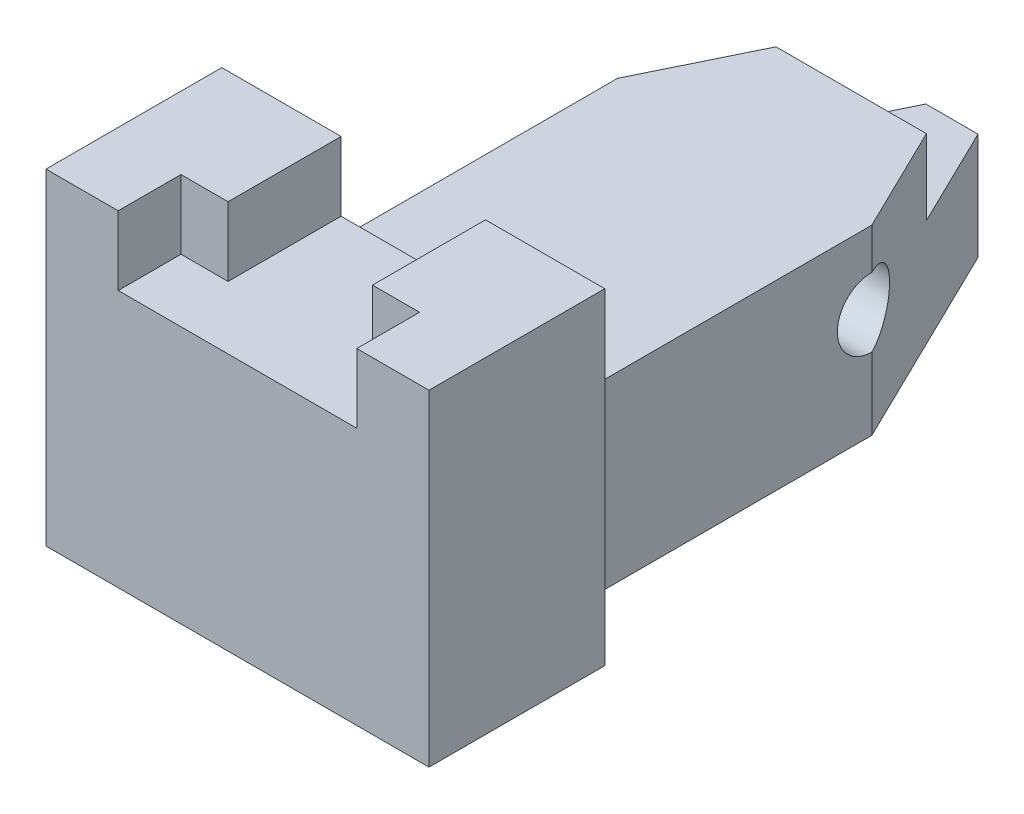
ISO-10303-21;
HEADER;
FILE_DESCRIPTION(('STEP AP214'),'2;1');
FILE_NAME('part.step','',(''),(''),'','','');
FILE_SCHEMA(('AUTOMOTIVE_DESIGN { 1 0 10303 214 1 1 1 1 }'));
ENDSEC;
DATA;
#1=APPLICATION_CONTEXT('core data for automotive mechanical design processes');
#2=APPLICATION_PROTOCOL_DEFINITION('international standard','automotive_design',2000,#1);
#3=PRODUCT_CONTEXT('',#1,'mechanical');
#4=PRODUCT('Part','Part','',(#3));
#5=PRODUCT_RELATED_PRODUCT_CATEGORY('part','',(#4));
#6=PRODUCT_DEFINITION_FORMATION('','',#4);
#7=PRODUCT_DEFINITION_CONTEXT('part definition',#1,'design');
#8=PRODUCT_DEFINITION('design','',#6,#7);
#9=PRODUCT_DEFINITION_SHAPE('','',#8);
#10=(LENGTH_UNIT() NAMED_UNIT(*) SI_UNIT(.MILLI.,.METRE.));
#11=(NAMED_UNIT(*) PLANE_ANGLE_UNIT() SI_UNIT($,.RADIAN.));
#12=(NAMED_UNIT(*) SI_UNIT($,.STERADIAN.) SOLID_ANGLE_UNIT());
#13=UNCERTAINTY_MEASURE_WITH_UNIT(LENGTH_MEASURE(1.E-05),#10,'distance_accuracy_value','');
#14=(GEOMETRIC_REPRESENTATION_CONTEXT(3) GLOBAL_UNCERTAINTY_ASSIGNED_CONTEXT((#13)) GLOBAL_UNIT_ASSIGNED_CONTEXT((#10,
#11,#12)) REPRESENTATION_CONTEXT('',''));
#15=CARTESIAN_POINT('',(0.,0.,0.));
#16=DIRECTION('',(0.,0.,1.));
#17=DIRECTION('',(1.,0.,0.));
#18=AXIS2_PLACEMENT_3D('',#15,#16,#17);
#19=CARTESIAN_POINT('',(-30.5,20.5,120.));
#20=DIRECTION('',(1.,0.,0.));
#21=DIRECTION('',(0.,1.,0.));
#22=AXIS2_PLACEMENT_3D('',#19,#20,#21);
#23=PLANE('',#22);
#24=DIRECTION('',(0.,1.,0.));
#25=VECTOR('',#24,1.);
#26=CARTESIAN_POINT('',(-30.5,20.5,92.));
#27=LINE('',#26,#25);
#28=CARTESIAN_POINT('',(-30.5,-20.5,92.));
#29=VERTEX_POINT('',#28);
#30=CARTESIAN_POINT('',(-30.5,31.5,92.));
#31=VERTEX_POINT('',#30);
#32=EDGE_CURVE('E341',#29,#31,#27,.T.);
#33=ORIENTED_EDGE('',*,*,#32,.F.);
#34=DIRECTION('',(0.,0.,-1.));
#35=VECTOR('',#34,1.);
#36=CARTESIAN_POINT('',(-30.5,-20.5,120.));
#37=LINE('',#36,#35);
#38=CARTESIAN_POINT('',(-30.5,-20.5,120.));
#39=VERTEX_POINT('',#38);
#40=EDGE_CURVE('E339',#39,#29,#37,.T.);
#41=ORIENTED_EDGE('',*,*,#40,.F.);
#42=DIRECTION('',(0.,-1.,0.));
#43=VECTOR('',#42,1.);
#44=CARTESIAN_POINT('',(-30.5,20.5,120.));
#45=LINE('',#44,#43);
#46=CARTESIAN_POINT('',(-30.5,31.5,120.));
#47=VERTEX_POINT('',#46);
#48=EDGE_CURVE('E335',#47,#39,#45,.T.);
#49=ORIENTED_EDGE('',*,*,#48,.F.);
#50=DIRECTION('',(0.,0.,1.));
#51=VECTOR('',#50,1.);
#52=CARTESIAN_POINT('',(-30.5,31.5,120.));
#53=LINE('',#52,#51);
#54=EDGE_CURVE('E254',#31,#47,#53,.T.);
#55=ORIENTED_EDGE('',*,*,#54,.F.);
#56=EDGE_LOOP('',(#33,#41,#49,#55));
#57=FACE_BOUND('',#56,.T.);
#58=ADVANCED_FACE('F41',(#57),#23,.F.);
#59=CARTESIAN_POINT('',(30.5,20.5,120.));
#60=DIRECTION('',(-1.,0.,0.));
#61=DIRECTION('',(0.,-1.,0.));
#62=AXIS2_PLACEMENT_3D('',#59,#60,#61);
#63=PLANE('',#62);
#64=DIRECTION('',(0.,0.,-1.));
#65=VECTOR('',#64,1.);
#66=CARTESIAN_POINT('',(30.5,-20.5,120.));
#67=LINE('',#66,#65);
#68=CARTESIAN_POINT('',(30.5,-20.5,120.));
#69=VERTEX_POINT('',#68);
#70=CARTESIAN_POINT('',(30.5,-20.5,92.));
#71=VERTEX_POINT('',#70);
#72=EDGE_CURVE('E337',#69,#71,#67,.T.);
#73=ORIENTED_EDGE('',*,*,#72,.T.);
#74=DIRECTION('',(0.,1.,0.));
#75=VECTOR('',#74,1.);
#76=CARTESIAN_POINT('',(30.5,0.,92.));
#77=LINE('',#76,#75);
#78=CARTESIAN_POINT('',(30.5,31.5,92.));
#79=VERTEX_POINT('',#78);
#80=EDGE_CURVE('E278',#71,#79,#77,.T.);
#81=ORIENTED_EDGE('',*,*,#80,.T.);
#82=DIRECTION('',(0.,0.,-1.));
#83=VECTOR('',#82,1.);
#84=CARTESIAN_POINT('',(30.5,31.5,92.));
#85=LINE('',#84,#83);
#86=CARTESIAN_POINT('',(30.5,31.5,120.));
#87=VERTEX_POINT('',#86);
#88=EDGE_CURVE('E305',#87,#79,#85,.T.);
#89=ORIENTED_EDGE('',*,*,#88,.F.);
#90=DIRECTION('',(0.,1.,0.));
#91=VECTOR('',#90,1.);
#92=CARTESIAN_POINT('',(30.5,20.5,120.));
#93=LINE('',#92,#91);
#94=EDGE_CURVE('E316',#69,#87,#93,.T.);
#95=ORIENTED_EDGE('',*,*,#94,.F.);
#96=EDGE_LOOP('',(#73,#81,#89,#95));
#97=FACE_BOUND('',#96,.T.);
#98=ADVANCED_FACE('F43',(#97),#63,.F.);
#99=CARTESIAN_POINT('',(-89.5,0.,22.));
#100=DIRECTION('',(0.,0.,-1.));
#101=DIRECTION('',(-1.,0.,0.));
#102=AXIS2_PLACEMENT_3D('',#99,#100,#101);
#103=PLANE('',#102);
#104=DIRECTION('',(1.,0.,0.));
#105=VECTOR('',#104,1.);
#106=CARTESIAN_POINT('',(-89.5,-3.50000000000002,22.));
#107=LINE('',#106,#105);
#108=CARTESIAN_POINT('',(-12.2301169484492,-3.50000000000001,22.));
#109=VERTEX_POINT('',#108);
#110=CARTESIAN_POINT('',(11.7239944957032,-3.50000000000001,22.));
#111=VERTEX_POINT('',#110);
#112=EDGE_CURVE('E318',#109,#111,#107,.T.);
#113=ORIENTED_EDGE('',*,*,#112,.F.);
#114=DIRECTION('',(0.,1.,0.));
#115=VECTOR('',#114,1.);
#116=CARTESIAN_POINT('',(-12.2301169484492,0.,22.));
#117=LINE('',#116,#115);
#118=CARTESIAN_POINT('',(-12.2301169484492,8.49999999999999,22.));
#119=VERTEX_POINT('',#118);
#120=EDGE_CURVE('E234',#109,#119,#117,.T.);
#121=ORIENTED_EDGE('',*,*,#120,.T.);
#122=DIRECTION('',(1.,0.,0.));
#123=VECTOR('',#122,1.);
#124=CARTESIAN_POINT('',(-89.5,8.49999999999998,22.));
#125=LINE('',#124,#123);
#126=CARTESIAN_POINT('',(11.7239944957032,8.5,22.));
#127=VERTEX_POINT('',#126);
#128=EDGE_CURVE('E325',#119,#127,#125,.T.);
#129=ORIENTED_EDGE('',*,*,#128,.T.);
#130=DIRECTION('',(0.,-1.,0.));
#131=VECTOR('',#130,1.);
#132=CARTESIAN_POINT('',(11.7239944957032,0.,22.));
#133=LINE('',#132,#131);
#134=EDGE_CURVE('E225',#127,#111,#133,.T.);
#135=ORIENTED_EDGE('',*,*,#134,.T.);
#136=EDGE_LOOP('',(#113,#121,#129,#135));
#137=FACE_BOUND('',#136,.T.);
#138=ADVANCED_FACE('F413',(#137),#103,.T.);
#139=CARTESIAN_POINT('',(-89.5,8.49999999999998,0.));
#140=DIRECTION('',(0.,1.,0.));
#141=DIRECTION('',(-1.,0.,0.));
#142=AXIS2_PLACEMENT_3D('',#139,#140,#141);
#143=PLANE('',#142);
#144=ORIENTED_EDGE('',*,*,#128,.F.);
#145=DIRECTION('',(-0.438371146789085,0.,0.898794046299164));
#146=VECTOR('',#145,1.);
#147=CARTESIAN_POINT('',(-18.4108950856716,8.49999999999999,34.6724731586962));
#148=LINE('',#147,#146);
#149=CARTESIAN_POINT('',(-20.5,8.49999999999999,38.9557729900058));
#150=VERTEX_POINT('',#149);
#151=EDGE_CURVE('E353',#119,#150,#148,.T.);
#152=ORIENTED_EDGE('',*,*,#151,.T.);
#153=DIRECTION('',(0.,0.,-1.));
#154=VECTOR('',#153,1.);
#155=CARTESIAN_POINT('',(-20.5,8.49999999999999,0.));
#156=LINE('',#155,#154);
#157=CARTESIAN_POINT('',(-20.5,8.49999999999998,92.));
#158=VERTEX_POINT('',#157);
#159=EDGE_CURVE('E198',#158,#150,#156,.T.);
#160=ORIENTED_EDGE('',*,*,#159,.F.);
#161=DIRECTION('',(1.,0.,0.));
#162=VECTOR('',#161,1.);
#163=CARTESIAN_POINT('',(-89.5,8.49999999999997,92.));
#164=LINE('',#163,#162);
#165=CARTESIAN_POINT('',(19.9938775472544,8.49999999999999,92.));
#166=VERTEX_POINT('',#165);
#167=EDGE_CURVE('E314',#158,#166,#164,.T.);
#168=ORIENTED_EDGE('',*,*,#167,.T.);
#169=DIRECTION('',(0.,0.,1.));
#170=VECTOR('',#169,1.);
#171=CARTESIAN_POINT('',(19.9938775472544,8.5,0.));
#172=LINE('',#171,#170);
#173=CARTESIAN_POINT('',(19.9938775472544,8.49999999999999,38.9557729900071));
#174=VERTEX_POINT('',#173);
#175=EDGE_CURVE('E342',#174,#166,#172,.T.);
#176=ORIENTED_EDGE('',*,*,#175,.F.);
#177=DIRECTION('',(-0.438371146789072,0.,-0.89879404629917));
#178=VECTOR('',#177,1.);
#179=CARTESIAN_POINT('',(-16.3962641470313,8.5,-35.6550743214029));
#180=LINE('',#179,#178);
#181=EDGE_CURVE('E350',#174,#127,#180,.T.);
#182=ORIENTED_EDGE('',*,*,#181,.T.);
#183=EDGE_LOOP('',(#144,#152,#160,#168,#176,#182));
#184=FACE_BOUND('',#183,.T.);
#185=ADVANCED_FACE('F407',(#184),#143,.T.);
#186=CARTESIAN_POINT('',(-30.5,20.5,120.));
#187=DIRECTION('',(0.,-1.,0.));
#188=DIRECTION('',(0.,0.,-1.));
#189=AXIS2_PLACEMENT_3D('',#186,#187,#188);
#190=PLANE('',#189);
#191=DIRECTION('',(0.,0.,-1.));
#192=VECTOR('',#191,1.);
#193=CARTESIAN_POINT('',(-19.,20.5,110.));
#194=LINE('',#193,#192);
#195=CARTESIAN_POINT('',(-19.,20.5,120.));
#196=VERTEX_POINT('',#195);
#197=CARTESIAN_POINT('',(-19.,20.5,110.));
#198=VERTEX_POINT('',#197);
#199=EDGE_CURVE('E258',#196,#198,#194,.T.);
#200=ORIENTED_EDGE('',*,*,#199,.F.);
#201=DIRECTION('',(-1.,0.,0.));
#202=VECTOR('',#201,1.);
#203=CARTESIAN_POINT('',(-30.5,20.5,120.));
#204=LINE('',#203,#202);
#205=CARTESIAN_POINT('',(19.,20.5,120.));
#206=VERTEX_POINT('',#205);
#207=EDGE_CURVE('E326',#206,#196,#204,.T.);
#208=ORIENTED_EDGE('',*,*,#207,.F.);
#209=DIRECTION('',(0.,0.,1.));
#210=VECTOR('',#209,1.);
#211=CARTESIAN_POINT('',(19.,20.5,120.));
#212=LINE('',#211,#210);
#213=CARTESIAN_POINT('',(19.,20.5,110.));
#214=VERTEX_POINT('',#213);
#215=EDGE_CURVE('E292',#214,#206,#212,.T.);
#216=ORIENTED_EDGE('',*,*,#215,.F.);
#217=DIRECTION('',(1.,0.,0.));
#218=VECTOR('',#217,1.);
#219=CARTESIAN_POINT('',(19.,20.5,110.));
#220=LINE('',#219,#218);
#221=CARTESIAN_POINT('',(11.5,20.5,110.));
#222=VERTEX_POINT('',#221);
#223=EDGE_CURVE('E294',#222,#214,#220,.T.);
#224=ORIENTED_EDGE('',*,*,#223,.F.);
#225=DIRECTION('',(0.,0.,1.));
#226=VECTOR('',#225,1.);
#227=CARTESIAN_POINT('',(11.5,20.5,110.));
#228=LINE('',#227,#226);
#229=CARTESIAN_POINT('',(11.5,20.5,92.));
#230=VERTEX_POINT('',#229);
#231=EDGE_CURVE('E264',#230,#222,#228,.T.);
#232=ORIENTED_EDGE('',*,*,#231,.F.);
#233=DIRECTION('',(1.,0.,0.));
#234=VECTOR('',#233,1.);
#235=CARTESIAN_POINT('',(-89.5,20.5,92.));
#236=LINE('',#235,#234);
#237=CARTESIAN_POINT('',(-11.5,20.5,92.));
#238=VERTEX_POINT('',#237);
#239=EDGE_CURVE('E317',#238,#230,#236,.T.);
#240=ORIENTED_EDGE('',*,*,#239,.F.);
#241=DIRECTION('',(0.,0.,-1.));
#242=VECTOR('',#241,1.);
#243=CARTESIAN_POINT('',(-11.5,20.5,92.));
#244=LINE('',#243,#242);
#245=CARTESIAN_POINT('',(-11.5,20.5,110.));
#246=VERTEX_POINT('',#245);
#247=EDGE_CURVE('E250',#246,#238,#244,.T.);
#248=ORIENTED_EDGE('',*,*,#247,.F.);
#249=DIRECTION('',(1.,0.,0.));
#250=VECTOR('',#249,1.);
#251=CARTESIAN_POINT('',(-11.5,20.5,110.));
#252=LINE('',#251,#250);
#253=EDGE_CURVE('E265',#198,#246,#252,.T.);
#254=ORIENTED_EDGE('',*,*,#253,.F.);
#255=EDGE_LOOP('',(#200,#208,#216,#224,#232,#240,#248,#254));
#256=FACE_BOUND('',#255,.T.);
#257=ADVANCED_FACE('F437',(#256),#190,.F.);
#258=CARTESIAN_POINT('',(-30.5,-20.5,120.));
#259=DIRECTION('',(0.,1.,0.));
#260=DIRECTION('',(0.,0.,1.));
#261=AXIS2_PLACEMENT_3D('',#258,#259,#260);
#262=PLANE('',#261);
#263=DIRECTION('',(-0.438371146789085,0.,0.898794046299164));
#264=VECTOR('',#263,1.);
#265=CARTESIAN_POINT('',(-54.353553824182,-20.5,108.365844446836));
#266=LINE('',#265,#264);
#267=CARTESIAN_POINT('',(-4.40482457732624,-20.5,5.95577299000578));
#268=VERTEX_POINT('',#267);
#269=CARTESIAN_POINT('',(-20.5,-20.5,38.9557729900058));
#270=VERTEX_POINT('',#269);
#271=EDGE_CURVE('E239',#268,#270,#266,.T.);
#272=ORIENTED_EDGE('',*,*,#271,.F.);
#273=DIRECTION('',(1.,0.,0.));
#274=VECTOR('',#273,1.);
#275=CARTESIAN_POINT('',(-30.4999999999997,-20.5,5.95577299000573));
#276=LINE('',#275,#274);
#277=CARTESIAN_POINT('',(3.89870212458057,-20.5,5.9557729900058));
#278=VERTEX_POINT('',#277);
#279=EDGE_CURVE('E47',#268,#278,#276,.T.);
#280=ORIENTED_EDGE('',*,*,#279,.T.);
#281=DIRECTION('',(-0.438371146789072,0.,-0.89879404629917));
#282=VECTOR('',#281,1.);
#283=CARTESIAN_POINT('',(42.2223675472644,-20.5,84.5309314295353));
#284=LINE('',#283,#282);
#285=CARTESIAN_POINT('',(19.9938775472544,-20.5,38.9557729900071));
#286=VERTEX_POINT('',#285);
#287=EDGE_CURVE('E226',#286,#278,#284,.T.);
#288=ORIENTED_EDGE('',*,*,#287,.F.);
#289=DIRECTION('',(0.,0.,1.));
#290=VECTOR('',#289,1.);
#291=CARTESIAN_POINT('',(19.9938775472544,-20.5,120.));
#292=LINE('',#291,#290);
#293=CARTESIAN_POINT('',(19.9938775472544,-20.5,92.));
#294=VERTEX_POINT('',#293);
#295=EDGE_CURVE('E216',#286,#294,#292,.T.);
#296=ORIENTED_EDGE('',*,*,#295,.T.);
#297=DIRECTION('',(-1.,0.,0.));
#298=VECTOR('',#297,1.);
#299=CARTESIAN_POINT('',(-30.5,-20.5,92.));
#300=LINE('',#299,#298);
#301=EDGE_CURVE('E351',#71,#294,#300,.T.);
#302=ORIENTED_EDGE('',*,*,#301,.F.);
#303=ORIENTED_EDGE('',*,*,#72,.F.);
#304=DIRECTION('',(1.,0.,0.));
#305=VECTOR('',#304,1.);
#306=CARTESIAN_POINT('',(-30.5,-20.5,120.));
#307=LINE('',#306,#305);
#308=EDGE_CURVE('E334',#39,#69,#307,.T.);
#309=ORIENTED_EDGE('',*,*,#308,.F.);
#310=ORIENTED_EDGE('',*,*,#40,.T.);
#311=DIRECTION('',(-1.,0.,0.));
#312=VECTOR('',#311,1.);
#313=CARTESIAN_POINT('',(-30.5,-20.5,92.));
#314=LINE('',#313,#312);
#315=CARTESIAN_POINT('',(-20.5,-20.5,92.));
#316=VERTEX_POINT('',#315);
#317=EDGE_CURVE('E352',#316,#29,#314,.T.);
#318=ORIENTED_EDGE('',*,*,#317,.F.);
#319=DIRECTION('',(0.,0.,-1.));
#320=VECTOR('',#319,1.);
#321=CARTESIAN_POINT('',(-20.5,-20.5,120.));
#322=LINE('',#321,#320);
#323=EDGE_CURVE('E233',#316,#270,#322,.T.);
#324=ORIENTED_EDGE('',*,*,#323,.T.);
#325=EDGE_LOOP('',(#272,#280,#288,#296,#302,#303,#309,#310,#318,#324));
#326=FACE_BOUND('',#325,.T.);
#327=ADVANCED_FACE('F363',(#326),#262,.F.);
#328=CARTESIAN_POINT('',(0.,0.,120.));
#329=DIRECTION('',(0.,0.,1.));
#330=DIRECTION('',(1.,0.,0.));
#331=AXIS2_PLACEMENT_3D('',#328,#329,#330);
#332=PLANE('',#331);
#333=ORIENTED_EDGE('',*,*,#94,.T.);
#334=DIRECTION('',(1.,0.,0.));
#335=VECTOR('',#334,1.);
#336=CARTESIAN_POINT('',(30.5,31.5,120.));
#337=LINE('',#336,#335);
#338=CARTESIAN_POINT('',(19.,31.5,120.));
#339=VERTEX_POINT('',#338);
#340=EDGE_CURVE('E304',#339,#87,#337,.T.);
#341=ORIENTED_EDGE('',*,*,#340,.F.);
#342=DIRECTION('',(0.,-1.,0.));
#343=VECTOR('',#342,1.);
#344=CARTESIAN_POINT('',(19.,31.5,120.));
#345=LINE('',#344,#343);
#346=EDGE_CURVE('E283',#339,#206,#345,.T.);
#347=ORIENTED_EDGE('',*,*,#346,.T.);
#348=ORIENTED_EDGE('',*,*,#207,.T.);
#349=DIRECTION('',(0.,-1.,0.));
#350=VECTOR('',#349,1.);
#351=CARTESIAN_POINT('',(-19.,31.5,120.));
#352=LINE('',#351,#350);
#353=CARTESIAN_POINT('',(-19.,31.5,120.));
#354=VERTEX_POINT('',#353);
#355=EDGE_CURVE('E260',#354,#196,#352,.T.);
#356=ORIENTED_EDGE('',*,*,#355,.F.);
#357=DIRECTION('',(1.,0.,0.));
#358=VECTOR('',#357,1.);
#359=CARTESIAN_POINT('',(-19.,31.5,120.));
#360=LINE('',#359,#358);
#361=EDGE_CURVE('E259',#47,#354,#360,.T.);
#362=ORIENTED_EDGE('',*,*,#361,.F.);
#363=ORIENTED_EDGE('',*,*,#48,.T.);
#364=ORIENTED_EDGE('',*,*,#308,.T.);
#365=EDGE_LOOP('',(#333,#341,#347,#348,#356,#362,#363,#364));
#366=FACE_BOUND('',#365,.T.);
#367=ADVANCED_FACE('F382',(#366),#332,.T.);
#368=CARTESIAN_POINT('',(-89.5,0.,92.));
#369=DIRECTION('',(0.,0.,-1.));
#370=DIRECTION('',(-1.,0.,0.));
#371=AXIS2_PLACEMENT_3D('',#368,#369,#370);
#372=PLANE('',#371);
#373=ORIENTED_EDGE('',*,*,#80,.F.);
#374=ORIENTED_EDGE('',*,*,#301,.T.);
#375=DIRECTION('',(0.,-1.,0.));
#376=VECTOR('',#375,1.);
#377=CARTESIAN_POINT('',(19.9938775472544,31.5,92.));
#378=LINE('',#377,#376);
#379=EDGE_CURVE('E208',#166,#294,#378,.T.);
#380=ORIENTED_EDGE('',*,*,#379,.F.);
#381=ORIENTED_EDGE('',*,*,#167,.F.);
#382=DIRECTION('',(0.,1.,0.));
#383=VECTOR('',#382,1.);
#384=CARTESIAN_POINT('',(-20.5,-51.,92.));
#385=LINE('',#384,#383);
#386=EDGE_CURVE('E205',#316,#158,#385,.T.);
#387=ORIENTED_EDGE('',*,*,#386,.F.);
#388=ORIENTED_EDGE('',*,*,#317,.T.);
#389=ORIENTED_EDGE('',*,*,#32,.T.);
#390=DIRECTION('',(-1.,0.,0.));
#391=VECTOR('',#390,1.);
#392=CARTESIAN_POINT('',(-30.5,31.5,92.));
#393=LINE('',#392,#391);
#394=CARTESIAN_POINT('',(-11.5,31.5,92.));
#395=VERTEX_POINT('',#394);
#396=EDGE_CURVE('E252',#395,#31,#393,.T.);
#397=ORIENTED_EDGE('',*,*,#396,.F.);
#398=DIRECTION('',(0.,-1.,0.));
#399=VECTOR('',#398,1.);
#400=CARTESIAN_POINT('',(-11.5,31.5,92.));
#401=LINE('',#400,#399);
#402=EDGE_CURVE('E267',#395,#238,#401,.T.);
#403=ORIENTED_EDGE('',*,*,#402,.T.);
#404=ORIENTED_EDGE('',*,*,#239,.T.);
#405=DIRECTION('',(0.,-1.,0.));
#406=VECTOR('',#405,1.);
#407=CARTESIAN_POINT('',(11.5,31.5,92.));
#408=LINE('',#407,#406);
#409=CARTESIAN_POINT('',(11.5,31.5,92.));
#410=VERTEX_POINT('',#409);
#411=EDGE_CURVE('E286',#410,#230,#408,.T.);
#412=ORIENTED_EDGE('',*,*,#411,.F.);
#413=DIRECTION('',(-1.,0.,0.));
#414=VECTOR('',#413,1.);
#415=CARTESIAN_POINT('',(11.5,31.5,92.));
#416=LINE('',#415,#414);
#417=EDGE_CURVE('E293',#79,#410,#416,.T.);
#418=ORIENTED_EDGE('',*,*,#417,.F.);
#419=EDGE_LOOP('',(#373,#374,#380,#381,#387,#388,#389,#397,#403,#404,#412,#418));
#420=FACE_BOUND('',#419,.T.);
#421=ADVANCED_FACE('F403',(#420),#372,.T.);
#422=CARTESIAN_POINT('',(-89.5,-3.50000000000002,0.));
#423=DIRECTION('',(0.,1.,0.));
#424=DIRECTION('',(-1.,0.,0.));
#425=AXIS2_PLACEMENT_3D('',#422,#423,#424);
#426=PLANE('',#425);
#427=DIRECTION('',(1.,0.,0.));
#428=VECTOR('',#427,1.);
#429=CARTESIAN_POINT('',(3.89870212458057,-3.5,5.9557729900058));
#430=LINE('',#429,#428);
#431=CARTESIAN_POINT('',(-4.40482457732625,-3.5,5.95577299000578));
#432=VERTEX_POINT('',#431);
#433=CARTESIAN_POINT('',(3.89870212458057,-3.5,5.9557729900058));
#434=VERTEX_POINT('',#433);
#435=EDGE_CURVE('E202',#432,#434,#430,.T.);
#436=ORIENTED_EDGE('',*,*,#435,.F.);
#437=DIRECTION('',(-0.438371146789085,0.,0.898794046299164));
#438=VECTOR('',#437,1.);
#439=CARTESIAN_POINT('',(-18.4108950856716,-3.50000000000001,34.6724731586962));
#440=LINE('',#439,#438);
#441=EDGE_CURVE('E240',#432,#109,#440,.T.);
#442=ORIENTED_EDGE('',*,*,#441,.T.);
#443=ORIENTED_EDGE('',*,*,#112,.T.);
#444=DIRECTION('',(-0.438371146789072,0.,-0.89879404629917));
#445=VECTOR('',#444,1.);
#446=CARTESIAN_POINT('',(-16.3962641470313,-3.5,-35.6550743214029));
#447=LINE('',#446,#445);
#448=EDGE_CURVE('E222',#111,#434,#447,.T.);
#449=ORIENTED_EDGE('',*,*,#448,.T.);
#450=EDGE_LOOP('',(#436,#442,#443,#449));
#451=FACE_BOUND('',#450,.T.);
#452=ADVANCED_FACE('F416',(#451),#426,.T.);
#453=CARTESIAN_POINT('',(11.5,31.5,110.));
#454=DIRECTION('',(1.,0.,0.));
#455=DIRECTION('',(0.,0.,-1.));
#456=AXIS2_PLACEMENT_3D('',#453,#454,#455);
#457=PLANE('',#456);
#458=ORIENTED_EDGE('',*,*,#231,.T.);
#459=DIRECTION('',(0.,-1.,0.));
#460=VECTOR('',#459,1.);
#461=CARTESIAN_POINT('',(11.5,31.5,110.));
#462=LINE('',#461,#460);
#463=CARTESIAN_POINT('',(11.5,31.5,110.));
#464=VERTEX_POINT('',#463);
#465=EDGE_CURVE('E245',#464,#222,#462,.T.);
#466=ORIENTED_EDGE('',*,*,#465,.F.);
#467=DIRECTION('',(0.,0.,1.));
#468=VECTOR('',#467,1.);
#469=CARTESIAN_POINT('',(11.5,31.5,110.));
#470=LINE('',#469,#468);
#471=EDGE_CURVE('E298',#410,#464,#470,.T.);
#472=ORIENTED_EDGE('',*,*,#471,.F.);
#473=ORIENTED_EDGE('',*,*,#411,.T.);
#474=EDGE_LOOP('',(#458,#466,#472,#473));
#475=FACE_BOUND('',#474,.T.);
#476=ADVANCED_FACE('F457',(#475),#457,.F.);
#477=CARTESIAN_POINT('',(19.,31.5,110.));
#478=DIRECTION('',(0.,0.,-1.));
#479=DIRECTION('',(-1.,0.,0.));
#480=AXIS2_PLACEMENT_3D('',#477,#478,#479);
#481=PLANE('',#480);
#482=ORIENTED_EDGE('',*,*,#223,.T.);
#483=DIRECTION('',(0.,-1.,0.));
#484=VECTOR('',#483,1.);
#485=CARTESIAN_POINT('',(19.,31.5,110.));
#486=LINE('',#485,#484);
#487=CARTESIAN_POINT('',(19.,31.5,110.));
#488=VERTEX_POINT('',#487);
#489=EDGE_CURVE('E285',#488,#214,#486,.T.);
#490=ORIENTED_EDGE('',*,*,#489,.F.);
#491=DIRECTION('',(1.,0.,0.));
#492=VECTOR('',#491,1.);
#493=CARTESIAN_POINT('',(19.,31.5,110.));
#494=LINE('',#493,#492);
#495=EDGE_CURVE('E309',#464,#488,#494,.T.);
#496=ORIENTED_EDGE('',*,*,#495,.F.);
#497=ORIENTED_EDGE('',*,*,#465,.T.);
#498=EDGE_LOOP('',(#482,#490,#496,#497));
#499=FACE_BOUND('',#498,.T.);
#500=ADVANCED_FACE('F456',(#499),#481,.F.);
#501=CARTESIAN_POINT('',(19.,31.5,120.));
#502=DIRECTION('',(1.,0.,0.));
#503=DIRECTION('',(0.,0.,-1.));
#504=AXIS2_PLACEMENT_3D('',#501,#502,#503);
#505=PLANE('',#504);
#506=ORIENTED_EDGE('',*,*,#215,.T.);
#507=ORIENTED_EDGE('',*,*,#346,.F.);
#508=DIRECTION('',(0.,0.,1.));
#509=VECTOR('',#508,1.);
#510=CARTESIAN_POINT('',(19.,31.5,120.));
#511=LINE('',#510,#509);
#512=EDGE_CURVE('E308',#488,#339,#511,.T.);
#513=ORIENTED_EDGE('',*,*,#512,.F.);
#514=ORIENTED_EDGE('',*,*,#489,.T.);
#515=EDGE_LOOP('',(#506,#507,#513,#514));
#516=FACE_BOUND('',#515,.T.);
#517=ADVANCED_FACE('F388',(#516),#505,.F.);
#518=CARTESIAN_POINT('',(0.,31.5,0.));
#519=DIRECTION('',(0.,-1.,0.));
#520=DIRECTION('',(0.,0.,-1.));
#521=AXIS2_PLACEMENT_3D('',#518,#519,#520);
#522=PLANE('',#521);
#523=ORIENTED_EDGE('',*,*,#471,.T.);
#524=ORIENTED_EDGE('',*,*,#495,.T.);
#525=ORIENTED_EDGE('',*,*,#512,.T.);
#526=ORIENTED_EDGE('',*,*,#340,.T.);
#527=ORIENTED_EDGE('',*,*,#88,.T.);
#528=ORIENTED_EDGE('',*,*,#417,.T.);
#529=EDGE_LOOP('',(#523,#524,#525,#526,#527,#528));
#530=FACE_BOUND('',#529,.T.);
#531=ADVANCED_FACE('F384',(#530),#522,.F.);
#532=CARTESIAN_POINT('',(-19.,31.5,110.));
#533=DIRECTION('',(-1.,0.,0.));
#534=DIRECTION('',(0.,0.,1.));
#535=AXIS2_PLACEMENT_3D('',#532,#533,#534);
#536=PLANE('',#535);
#537=ORIENTED_EDGE('',*,*,#199,.T.);
#538=DIRECTION('',(0.,-1.,0.));
#539=VECTOR('',#538,1.);
#540=CARTESIAN_POINT('',(-19.,31.5,110.));
#541=LINE('',#540,#539);
#542=CARTESIAN_POINT('',(-19.,31.5,110.));
#543=VERTEX_POINT('',#542);
#544=EDGE_CURVE('E279',#543,#198,#541,.T.);
#545=ORIENTED_EDGE('',*,*,#544,.F.);
#546=DIRECTION('',(0.,0.,-1.));
#547=VECTOR('',#546,1.);
#548=CARTESIAN_POINT('',(-19.,31.5,110.));
#549=LINE('',#548,#547);
#550=EDGE_CURVE('E243',#354,#543,#549,.T.);
#551=ORIENTED_EDGE('',*,*,#550,.F.);
#552=ORIENTED_EDGE('',*,*,#355,.T.);
#553=EDGE_LOOP('',(#537,#545,#551,#552));
#554=FACE_BOUND('',#553,.T.);
#555=ADVANCED_FACE('F393',(#554),#536,.F.);
#556=CARTESIAN_POINT('',(-11.5,31.5,110.));
#557=DIRECTION('',(0.,0.,-1.));
#558=DIRECTION('',(-1.,0.,0.));
#559=AXIS2_PLACEMENT_3D('',#556,#557,#558);
#560=PLANE('',#559);
#561=ORIENTED_EDGE('',*,*,#253,.T.);
#562=DIRECTION('',(0.,-1.,0.));
#563=VECTOR('',#562,1.);
#564=CARTESIAN_POINT('',(-11.5,31.5,110.));
#565=LINE('',#564,#563);
#566=CARTESIAN_POINT('',(-11.5,31.5,110.));
#567=VERTEX_POINT('',#566);
#568=EDGE_CURVE('E271',#567,#246,#565,.T.);
#569=ORIENTED_EDGE('',*,*,#568,.F.);
#570=DIRECTION('',(1.,0.,0.));
#571=VECTOR('',#570,1.);
#572=CARTESIAN_POINT('',(-11.5,31.5,110.));
#573=LINE('',#572,#571);
#574=EDGE_CURVE('E246',#543,#567,#573,.T.);
#575=ORIENTED_EDGE('',*,*,#574,.F.);
#576=ORIENTED_EDGE('',*,*,#544,.T.);
#577=EDGE_LOOP('',(#561,#569,#575,#576));
#578=FACE_BOUND('',#577,.T.);
#579=ADVANCED_FACE('F449',(#578),#560,.F.);
#580=CARTESIAN_POINT('',(-11.5,31.5,92.));
#581=DIRECTION('',(-1.,0.,0.));
#582=DIRECTION('',(0.,0.,1.));
#583=AXIS2_PLACEMENT_3D('',#580,#581,#582);
#584=PLANE('',#583);
#585=ORIENTED_EDGE('',*,*,#247,.T.);
#586=ORIENTED_EDGE('',*,*,#402,.F.);
#587=DIRECTION('',(0.,0.,-1.));
#588=VECTOR('',#587,1.);
#589=CARTESIAN_POINT('',(-11.5,31.5,92.));
#590=LINE('',#589,#588);
#591=EDGE_CURVE('E248',#567,#395,#590,.T.);
#592=ORIENTED_EDGE('',*,*,#591,.F.);
#593=ORIENTED_EDGE('',*,*,#568,.T.);
#594=EDGE_LOOP('',(#585,#586,#592,#593));
#595=FACE_BOUND('',#594,.T.);
#596=ADVANCED_FACE('F451',(#595),#584,.F.);
#597=CARTESIAN_POINT('',(0.,31.5,0.));
#598=DIRECTION('',(0.,-1.,0.));
#599=DIRECTION('',(0.,0.,-1.));
#600=AXIS2_PLACEMENT_3D('',#597,#598,#599);
#601=PLANE('',#600);
#602=ORIENTED_EDGE('',*,*,#550,.T.);
#603=ORIENTED_EDGE('',*,*,#574,.T.);
#604=ORIENTED_EDGE('',*,*,#591,.T.);
#605=ORIENTED_EDGE('',*,*,#396,.T.);
#606=ORIENTED_EDGE('',*,*,#54,.T.);
#607=ORIENTED_EDGE('',*,*,#361,.T.);
#608=EDGE_LOOP('',(#602,#603,#604,#605,#606,#607));
#609=FACE_BOUND('',#608,.T.);
#610=ADVANCED_FACE('F396',(#609),#601,.F.);
#611=CARTESIAN_POINT('',(0.80288483214509,31.5,-0.391593097502386));
#612=DIRECTION('',(0.89879404629917,0.,-0.438371146789072));
#613=DIRECTION('',(-0.438371146789072,0.,-0.89879404629917));
#614=AXIS2_PLACEMENT_3D('',#611,#612,#613);
#615=PLANE('',#614);
#616=CARTESIAN_POINT('',(19.9938775472544,-3.5,38.9557729900071));
#617=DIRECTION('',(0.89879404629917,0.,-0.438371146789072));
#618=DIRECTION('',(0.438371146789072,0.,0.89879404629917));
#619=AXIS2_PLACEMENT_3D('',#616,#617,#618);
#620=ELLIPSE('',#619,6.11931067261352,5.5);
#621=CARTESIAN_POINT('',(19.9938775472544,-9.,38.9557729900071));
#622=VERTEX_POINT('',#621);
#623=CARTESIAN_POINT('',(19.9938775472544,1.99999999999999,38.9557729900071));
#624=VERTEX_POINT('',#623);
#625=EDGE_CURVE('E54',#622,#624,#620,.T.);
#626=ORIENTED_EDGE('',*,*,#625,.F.);
#627=DIRECTION('',(0.,-1.,0.));
#628=VECTOR('',#627,1.);
#629=CARTESIAN_POINT('',(19.9938775472544,31.5,38.9557729900071));
#630=LINE('',#629,#628);
#631=EDGE_CURVE('E215',#622,#286,#630,.T.);
#632=ORIENTED_EDGE('',*,*,#631,.T.);
#633=ORIENTED_EDGE('',*,*,#287,.T.);
#634=DIRECTION('',(0.,-1.,0.));
#635=VECTOR('',#634,1.);
#636=CARTESIAN_POINT('',(3.89870212458057,31.5,5.9557729900058));
#637=LINE('',#636,#635);
#638=EDGE_CURVE('E220',#434,#278,#637,.T.);
#639=ORIENTED_EDGE('',*,*,#638,.F.);
#640=ORIENTED_EDGE('',*,*,#448,.F.);
#641=ORIENTED_EDGE('',*,*,#134,.F.);
#642=ORIENTED_EDGE('',*,*,#181,.F.);
#643=EDGE_CURVE('E213',#174,#624,#630,.T.);
#644=ORIENTED_EDGE('',*,*,#643,.T.);
#645=EDGE_LOOP('',(#626,#632,#633,#639,#640,#641,#642,#644));
#646=FACE_BOUND('',#645,.T.);
#647=ADVANCED_FACE('F366',(#646),#615,.T.);
#648=CARTESIAN_POINT('',(19.9938775472544,31.5,0.));
#649=DIRECTION('',(-1.,0.,0.));
#650=DIRECTION('',(0.,0.,1.));
#651=AXIS2_PLACEMENT_3D('',#648,#649,#650);
#652=PLANE('',#651);
#653=ORIENTED_EDGE('',*,*,#631,.F.);
#654=CARTESIAN_POINT('',(19.9938775472544,-3.5,38.9557729900071));
#655=DIRECTION('',(-1.,0.,0.));
#656=DIRECTION('',(0.,0.,1.));
#657=AXIS2_PLACEMENT_3D('',#654,#655,#656);
#658=CIRCLE('',#657,5.5);
#659=EDGE_CURVE('E197',#622,#624,#658,.T.);
#660=ORIENTED_EDGE('',*,*,#659,.T.);
#661=ORIENTED_EDGE('',*,*,#643,.F.);
#662=ORIENTED_EDGE('',*,*,#175,.T.);
#663=ORIENTED_EDGE('',*,*,#379,.T.);
#664=ORIENTED_EDGE('',*,*,#295,.F.);
#665=EDGE_LOOP('',(#653,#660,#661,#662,#663,#664));
#666=FACE_BOUND('',#665,.T.);
#667=ADVANCED_FACE('F369',(#666),#652,.F.);
#668=CARTESIAN_POINT('',(-1.21174610649425,-51.,-0.591008065205056));
#669=DIRECTION('',(-0.898794046299163,0.,-0.438371146789084));
#670=DIRECTION('',(-0.438371146789085,0.,0.898794046299164));
#671=AXIS2_PLACEMENT_3D('',#668,#669,#670);
#672=PLANE('',#671);
#673=CARTESIAN_POINT('',(-20.5000000000007,-3.5,38.9557729900071));
#674=DIRECTION('',(-0.898794046299163,0.,-0.438371146789084));
#675=DIRECTION('',(0.438371146789085,0.,-0.898794046299164));
#676=AXIS2_PLACEMENT_3D('',#673,#674,#675);
#677=ELLIPSE('',#676,6.11931067261356,5.5);
#678=CARTESIAN_POINT('',(-20.5,1.99999999999999,38.9557729900058));
#679=VERTEX_POINT('',#678);
#680=CARTESIAN_POINT('',(-20.5,-9.,38.9557729900058));
#681=VERTEX_POINT('',#680);
#682=EDGE_CURVE('E61',#679,#681,#677,.T.);
#683=ORIENTED_EDGE('',*,*,#682,.F.);
#684=DIRECTION('',(0.,1.,0.));
#685=VECTOR('',#684,1.);
#686=CARTESIAN_POINT('',(-20.5,-51.,38.9557729900058));
#687=LINE('',#686,#685);
#688=EDGE_CURVE('E195',#679,#150,#687,.T.);
#689=ORIENTED_EDGE('',*,*,#688,.T.);
#690=ORIENTED_EDGE('',*,*,#151,.F.);
#691=ORIENTED_EDGE('',*,*,#120,.F.);
#692=ORIENTED_EDGE('',*,*,#441,.F.);
#693=DIRECTION('',(0.,1.,0.));
#694=VECTOR('',#693,1.);
#695=CARTESIAN_POINT('',(-4.40482457732625,-51.,5.9557729900058));
#696=LINE('',#695,#694);
#697=EDGE_CURVE('E204',#268,#432,#696,.T.);
#698=ORIENTED_EDGE('',*,*,#697,.F.);
#699=ORIENTED_EDGE('',*,*,#271,.T.);
#700=EDGE_CURVE('E192',#270,#681,#687,.T.);
#701=ORIENTED_EDGE('',*,*,#700,.T.);
#702=EDGE_LOOP('',(#683,#689,#690,#691,#692,#698,#699,#701));
#703=FACE_BOUND('',#702,.T.);
#704=ADVANCED_FACE('F191',(#703),#672,.T.);
#705=CARTESIAN_POINT('',(-20.5,-51.,0.));
#706=DIRECTION('',(1.,0.,0.));
#707=DIRECTION('',(0.,0.,-1.));
#708=AXIS2_PLACEMENT_3D('',#705,#706,#707);
#709=PLANE('',#708);
#710=ORIENTED_EDGE('',*,*,#688,.F.);
#711=CARTESIAN_POINT('',(-20.5,-3.5,38.9557729900071));
#712=DIRECTION('',(1.,0.,0.));
#713=DIRECTION('',(0.,0.,-1.));
#714=AXIS2_PLACEMENT_3D('',#711,#712,#713);
#715=CIRCLE('',#714,5.5);
#716=EDGE_CURVE('E11',#679,#681,#715,.T.);
#717=ORIENTED_EDGE('',*,*,#716,.T.);
#718=ORIENTED_EDGE('',*,*,#700,.F.);
#719=ORIENTED_EDGE('',*,*,#323,.F.);
#720=ORIENTED_EDGE('',*,*,#386,.T.);
#721=ORIENTED_EDGE('',*,*,#159,.T.);
#722=EDGE_LOOP('',(#710,#717,#718,#719,#720,#721));
#723=FACE_BOUND('',#722,.T.);
#724=ADVANCED_FACE('F199',(#723),#709,.F.);
#725=CARTESIAN_POINT('',(3.89870212458058,-54.5,5.95577299000579));
#726=DIRECTION('',(0.,0.,1.));
#727=DIRECTION('',(1.,0.,0.));
#728=AXIS2_PLACEMENT_3D('',#725,#726,#727);
#729=PLANE('',#728);
#730=ORIENTED_EDGE('',*,*,#638,.T.);
#731=ORIENTED_EDGE('',*,*,#279,.F.);
#732=ORIENTED_EDGE('',*,*,#697,.T.);
#733=ORIENTED_EDGE('',*,*,#435,.T.);
#734=EDGE_LOOP('',(#730,#731,#732,#733));
#735=FACE_BOUND('',#734,.T.);
#736=ADVANCED_FACE('F419',(#735),#729,.F.);
#737=CARTESIAN_POINT('',(-30.5,-3.5,38.9557729900071));
#738=DIRECTION('',(1.,0.,0.));
#739=DIRECTION('',(0.,0.,-1.));
#740=AXIS2_PLACEMENT_3D('',#737,#738,#739);
#741=CYLINDRICAL_SURFACE('',#740,5.5);
#742=ORIENTED_EDGE('',*,*,#625,.T.);
#743=ORIENTED_EDGE('',*,*,#659,.F.);
#744=EDGE_LOOP('',(#742,#743));
#745=FACE_BOUND('',#744,.T.);
#746=ORIENTED_EDGE('',*,*,#682,.T.);
#747=ORIENTED_EDGE('',*,*,#716,.F.);
#748=EDGE_LOOP('',(#746,#747));
#749=FACE_BOUND('',#748,.T.);
#750=ADVANCED_FACE('F187',(#745,#749),#741,.F.);
#751=CLOSED_SHELL('',(#58,#98,#138,#185,#257,#327,#367,#421,#452,#476,#500,#517,#531,#555,#579,
#596,#610,#647,#667,#704,#724,#736,#750));
#752=MANIFOLD_SOLID_BREP('B2',#751);
#753=ADVANCED_BREP_SHAPE_REPRESENTATION('',(#18,#752),#14);
#754=SHAPE_DEFINITION_REPRESENTATION(#9,#753);
ENDSEC;
END-ISO-10303-21;
